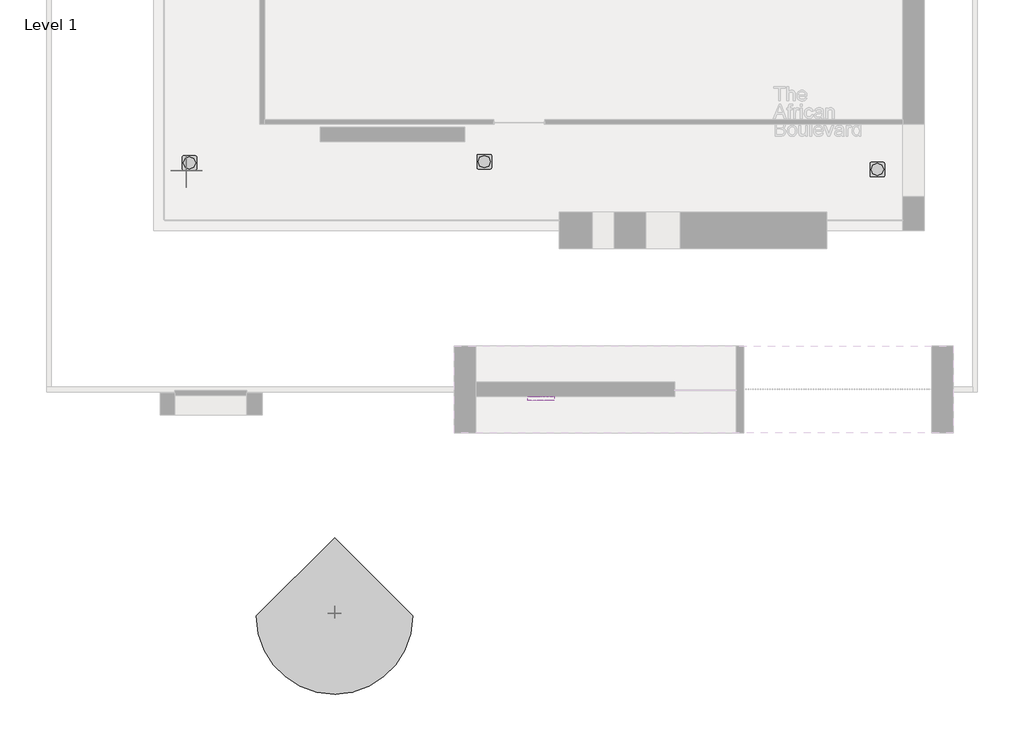
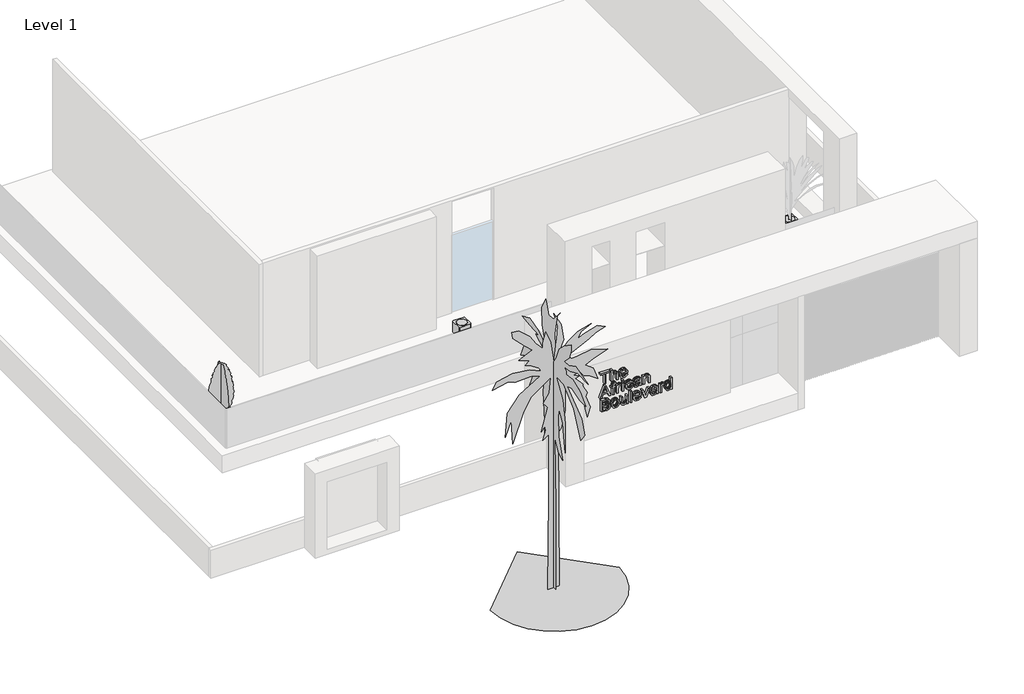
# One storey, part 2 of 3: 4 proxies, 2 geographic elements.
"""IFC4 building model written with IfcOpenShell, lengths in millimetres."""

from ifc_helpers import new_model, si_unit, frame, origin, place, context, project, spatial, polyline, outline, extrude, transform, mapped, element, save
from components import proxy_13b82c07, rpc_tree_conifer_chinese_juniper_7_5155a079, rpc_tree_tropical_cuban_royal_palm_25_0a7aa95b

model = new_model("IFC4")

# Units and contexts
model_context = context("Model", 3, world=origin())
ifc_project = project(units=[si_unit("LENGTHUNIT", "METRE", prefix="MILLI")], contexts=[model_context])

# Site, building, storey
site = spatial("IfcSite", under=ifc_project)
building = spatial("IfcBuilding", under=site)
storey = spatial("IfcBuildingStorey", under=building, Name="Level 1", Elevation=0.0)

# Proxies
placement = place(None, origin())
element("IfcBuildingElementProxy", 1, Name="24\" Arial", ObjectType="24\" Arial", at=placement, inside=storey, context=model_context, shape_type="SweptSolid", body=[
    extrude(outline(polyline([(2851.6933185, -10689.1512107), (2851.6933185, -10614.1235184), (3376.8871646, -10614.1235184), (3376.8871646, -10417.1758261), (3451.9148569, -10417.1758261), (3451.9148569, -10886.098903), (3376.8871646, -10886.098903), (3376.8871646, -10689.1512107), (2851.6933185, -10689.1512107)])), frame((0.0, -12620.7632813, 0.0), z_axis=(0.0, 1.0, 0.0), x_axis=(0.0, 0.0, 1.0)), (0.0, 0.0, 1.0), 152.4),
    extrude(outline(polyline([(2851.6933185, -10342.1481338), (2851.6933185, -10267.1204415), (3085.86178, -10267.1204415), (3130.8124531, -10264.0614511), (3164.8460108, -10254.88448), (3190.4536069, -10238.5088069), (3210.1263954, -10213.8537107), (3222.6554339, -10184.0880857), (3226.83178, -10152.3808261), (3225.2839675, -10131.718903), (3220.64053, -10113.5481338), (3212.9014675, -10097.8685184), (3202.06678, -10084.6800569), (3187.8342319, -10074.2300329), (3169.9015877, -10066.76573), (3148.2688473, -10062.2871482), (3122.9360108, -10060.7942877), (2851.6933185, -10060.7942877), (2851.6933185, -9985.7665954), (3130.7025493, -9985.7665954), (3187.6693762, -9989.61323), (3229.3229339, -10001.1531338), (3259.6380781, -10021.6318838), (3282.5896646, -10052.2950569), (3297.0420204, -10091.237653), (3301.8594723, -10136.5546723), (3297.4450012, -10174.2791675), (3284.2015877, -10208.6149607), (3262.1292319, -10239.5620521), (3231.2279339, -10267.1204415), (3451.9148569, -10267.1204415), (3451.9148569, -10342.1481338), (2851.6933185, -10342.1481338)])), frame((0.0, -12620.7632813, 0.0), z_axis=(0.0, 1.0, 0.0), x_axis=(0.0, 0.0, 1.0)), (0.0, 0.0, 1.0), 152.4),
    extrude(outline(polyline([(2982.99178, -9573.9935184), (2953.3543762, -9595.0217877), (2933.0221646, -9622.3512107), (2921.2624531, -9655.9817877), (2917.3425493, -9695.9135184), (2919.4581983, -9723.6596603), (2925.8051454, -9749.0153934), (2936.3833906, -9771.9807179), (2951.1929339, -9792.5556338), (2969.9773329, -9809.787641), (2992.4801454, -9822.7242396), (3018.7013714, -9831.3654295), (3048.6410108, -9835.7112107), (3048.6410108, -9498.5262107), (3068.8633185, -9498.0865954), (3121.1500733, -9501.6447324), (3167.2272608, -9512.3191434), (3207.094881, -9530.1098285), (3240.7529339, -9555.0167877), (3267.4870444, -9585.5288429), (3286.5828377, -9620.1348165), (3298.0403137, -9658.8347083), (3301.8594723, -9701.6285184), (3298.031155, -9745.8464992), (3286.5462031, -9785.7415954), (3267.4046166, -9821.3138069), (3240.6063954, -9852.5631338), (3206.8750733, -9878.0150329), (3166.9341839, -9896.1949607), (3120.7837271, -9907.1029175), (3068.4237031, -9910.738903), (3017.7809267, -9907.1395521), (2973.1187512, -9896.3414992), (2934.4371767, -9878.3447444), (2901.7362031, -9853.1492877), (2875.7393642, -9821.8175329), (2857.1701935, -9785.4118838), (2846.0286911, -9743.9323405), (2842.3148569, -9697.378903), (2844.4671406, -9660.1352372), (2850.9239916, -9626.3627011), (2861.6854098, -9596.0612949), (2876.7513954, -9569.2310184), (2895.7189675, -9546.1099968), (2918.1851454, -9526.936355), (2944.1499291, -9511.7100929), (2973.6133185, -9500.4312107), (2982.99178, -9573.9935184)]), holes=[polyline([(3123.6687031, -9835.7112107), (3146.0020805, -9831.6401891), (3165.9633666, -9823.3836627), (3183.5525613, -9810.9416314), (3198.7696646, -9794.3140954), (3211.0468401, -9774.4993478), (3219.8162512, -9752.4956819), (3225.0778978, -9728.3030978), (3226.83178, -9701.9215954), (3224.6337031, -9672.9985665), (3218.0394723, -9646.896403), (3207.0490877, -9623.615105), (3191.6625493, -9603.1546723), (3178.8953858, -9591.9902732), (3163.3073569, -9583.2620761), (3123.6687031, -9573.1142877), (3123.6687031, -9835.7112107)])]), frame((0.0, -12620.7632813, 0.0), z_axis=(0.0, 1.0, 0.0), x_axis=(0.0, 0.0, 1.0)), (0.0, 0.0, 1.0), 152.4),
    extrude(outline(polyline([(2110.7948569, -10908.958903), (2110.7948569, -10829.8281338), (2298.3640877, -10761.2481338), (2298.3640877, -10513.8912107), (2110.7948569, -10445.3112107), (2110.7948569, -10366.033903), (2711.0163954, -10605.4777492), (2711.0163954, -10669.3685184), (2110.7948569, -10908.958903)]), holes=[polyline([(2373.39178, -10733.698903), (2533.8513954, -10674.93698), (2635.9887031, -10637.5696723), (2520.9560108, -10595.5131338), (2373.39178, -10541.293903), (2373.39178, -10733.698903)])]), frame((0.0, -12620.7632813, 0.0), z_axis=(0.0, 1.0, 0.0), x_axis=(0.0, 0.0, 1.0)), (0.0, 0.0, 1.0), 152.4),
    extrude(outline(polyline([(2110.7948569, -10276.498903), (2110.7948569, -10201.4712107), (2476.5548569, -10201.4712107), (2476.5548569, -10117.0650569), (2551.5825493, -10117.0650569), (2551.5825493, -10201.4712107), (2586.4587031, -10201.4712107), (2615.0703377, -10198.0092396), (2632.9113954, -10187.6233261), (2642.2532223, -10168.8847204), (2645.3671646, -10140.3646723), (2641.8502416, -10097.1358261), (2712.1887031, -10086.1454415), (2718.3433185, -10122.01073), (2720.3948569, -10154.578903), (2716.1086069, -10197.5879415), (2703.2498569, -10230.1927492), (2683.5037993, -10253.4923646), (2658.5556262, -10268.5858261), (2632.7282223, -10274.5206338), (2595.9837031, -10276.498903), (2551.5825493, -10276.498903), (2551.5825493, -10342.1481338), (2476.5548569, -10342.1481338), (2476.5548569, -10276.498903), (2110.7948569, -10276.498903)])), frame((0.0, -12620.7632813, 0.0), z_axis=(0.0, 1.0, 0.0), x_axis=(0.0, 0.0, 1.0)), (0.0, 0.0, 1.0), 152.4),
    extrude(outline(polyline([(2110.7948569, -10051.4158261), (2110.7948569, -9976.3881338), (2342.4721646, -9976.3881338), (2388.1921646, -9973.3474607), (2430.1021646, -9964.2254415), (2453.4750493, -9953.363278), (2471.1329339, -9937.1890954), (2482.2332223, -9917.168278), (2485.9333185, -9894.7662107), (2482.0866839, -9868.3892877), (2470.54678, -9842.0123646), (2537.8079339, -9816.9542877), (2555.1727416, -9854.9077492), (2560.9610108, -9892.2750569), (2557.3341839, -9916.74698), (2546.4537031, -9939.1673646), (2524.1798569, -9961.51448), (2486.3729339, -9985.7665954), (2551.5825493, -9985.7665954), (2551.5825493, -10051.4158261), (2110.7948569, -10051.4158261)])), frame((0.0, -12620.7632813, 0.0), z_axis=(0.0, 1.0, 0.0), x_axis=(0.0, 0.0, 1.0)), (0.0, 0.0, 1.0), 152.4),
    extrude(outline(polyline([(-9695.0342877, -12620.7632813), (-9770.06198, -12620.7632813), (-9770.06198, -12468.3632813), (-9695.0342877, -12468.3632813), (-9695.0342877, -12620.7632813)])), frame((0.0, 0.0, 2110.7948569), z_axis=(0.0, 0.0, 1.0), x_axis=(1.0, 0.0, 0.0)), (0.0, 0.0, 1.0), 440.7876923),
    extrude(outline(polyline([(-9695.0342877, -12620.7632813), (-9770.06198, -12620.7632813), (-9770.06198, -12468.3632813), (-9695.0342877, -12468.3632813), (-9695.0342877, -12620.7632813)])), frame((0.0, 0.0, 2635.9887031), z_axis=(0.0, 0.0, 1.0), x_axis=(1.0, 0.0, 0.0)), (0.0, 0.0, 1.0), 75.0276923),
    extrude(outline(polyline([(2270.2287031, -9301.138903), (2247.8907464, -9306.2448526), (2228.6484146, -9313.9427011), (2212.5017079, -9324.2324487), (2199.4506262, -9337.1140954), (2189.3852656, -9352.1663429), (2182.1957223, -9368.9678934), (2176.4440877, -9407.818903), (2178.7474892, -9433.0097804), (2185.6576935, -9455.682028), (2197.1747007, -9475.8356458), (2213.2985108, -9493.4706338), (2234.5145324, -9507.7993478), (2261.3081743, -9518.0341434), (2293.6794363, -9524.1750208), (2331.6283185, -9526.22198), (2369.0139435, -9524.1292276), (2401.01428, -9517.8509704), (2427.6293281, -9507.3872083), (2448.8590877, -9492.7379415), (2465.0790637, -9474.745766), (2476.6647608, -9454.253278), (2483.6161791, -9431.2604776), (2485.9333185, -9405.7673646), (2481.2257704, -9372.9244319), (2467.1031262, -9345.3202492), (2443.638655, -9324.1271242), (2410.9056262, -9310.5173646), (2420.2840877, -9235.4896723), (2452.0646166, -9243.7095641), (2479.9985108, -9255.9134704), (2504.0857704, -9272.101391), (2524.3263954, -9292.2733261), (2540.3540396, -9316.0262949), (2551.8023569, -9342.9573165), (2558.6713473, -9373.066391), (2560.9610108, -9406.3535184), (2559.2941358, -9433.3944439), (2554.2935108, -9459.4187588), (2545.9591358, -9484.4264631), (2534.2910108, -9508.4175569), (2519.2845565, -9530.3983261), (2500.9351935, -9549.3750569), (2479.2429218, -9565.3477492), (2454.2077416, -9578.316403), (2426.3883305, -9588.3497083), (2396.3433666, -9595.516355), (2329.57678, -9601.2496723), (2277.679268, -9597.8930256), (2232.183655, -9587.8230857), (2193.0899411, -9571.0398526), (2160.3981262, -9547.5433261), (2134.593619, -9518.5149728), (2116.1618281, -9485.1362588), (2105.1027536, -9447.4071843), (2101.4163954, -9405.3277492), (2104.058667, -9371.4590473), (2111.9854819, -9340.3379415), (2125.1968401, -9311.9644319), (2143.6927416, -9286.3385184), (2166.8687151, -9264.3852252), (2194.1202896, -9247.0295761), (2225.4474651, -9234.2715713), (2260.8502416, -9226.1112107), (2270.2287031, -9301.138903)])), frame((0.0, -12620.7632813, 0.0), z_axis=(0.0, 1.0, 0.0), x_axis=(0.0, 0.0, 1.0)), (0.0, 0.0, 1.0), 152.4),
    extrude(outline(polyline([(2167.0656262, -8879.1081338), (2136.8787031, -8872.3673646), (2110.7948569, -8860.3512107), (2110.7948569, -8785.3235184), (2141.6595204, -8794.6287107), (2173.8796646, -8800.2704415), (2304.2256262, -8804.0804415), (2397.5706262, -8804.0804415), (2463.2198569, -8807.743903), (2491.3369243, -8816.792653), (2514.1419723, -8830.7504415), (2532.5875012, -8851.797028), (2547.6260108, -8882.1121723), (2557.6272608, -8922.3186627), (2560.9610108, -8973.0392877), (2557.1876454, -9025.921355), (2545.8675493, -9072.0260184), (2527.5868762, -9109.7230377), (2502.93178, -9137.3821723), (2470.6933185, -9156.8168357), (2429.6625493, -9169.8404415), (2420.2840877, -9094.8127492), (2451.4784627, -9079.9024607), (2471.49928, -9058.6177492), (2482.3248089, -9027.4050569), (2485.9333185, -8982.7108261), (2480.5113954, -8934.426403), (2473.7339916, -8915.3947204), (2464.2456262, -8899.7700569), (2454.7389435, -8890.7304655), (2442.3381262, -8884.2736146), (2408.8540877, -8879.1081338), (2392.1487031, -8879.5477492), (2378.2275493, -8932.9610184), (2366.3579339, -9009.673903), (2355.0744723, -9074.5904415), (2344.7435108, -9102.304528), (2330.4560108, -9127.12448), (2311.5525493, -9148.2443357), (2287.3737031, -9164.8581338), (2259.1284146, -9175.6287107), (2228.0256262, -9179.218903), (2201.5662752, -9176.8422324), (2177.5797608, -9169.7122204), (2156.0660829, -9157.828867), (2137.0252416, -9141.1921723), (2121.4463714, -9120.1226891), (2110.3186069, -9094.9409704), (2103.6419483, -9065.647016), (2101.4163954, -9032.2408261), (2105.1164916, -8990.678855), (2116.21678, -8951.86448), (2136.3291839, -8914.955105), (2167.0656262, -8879.1081338)]), holes=[polyline([(2317.1210108, -8879.1081338), (2295.8729339, -8879.5477492), (2262.1690877, -8882.515153), (2237.8437031, -8891.4173646), (2214.2326935, -8911.4931338), (2194.3950493, -8940.3612107), (2180.9318281, -8975.9700569), (2176.4440877, -9016.2681338), (2180.51053, -9054.2765473), (2192.7098569, -9081.8440954), (2210.99053, -9098.6044319), (2233.3010108, -9104.1912107), (2248.4311069, -9101.6267877), (2262.1690877, -9093.9335184), (2273.6357223, -9081.4960665), (2281.95178, -9064.6990954), (2294.1144723, -9000.148903), (2304.6286069, -8929.5173646), (2317.1210108, -8879.1081338)])]), frame((0.0, -12620.7632813, 0.0), z_axis=(0.0, 1.0, 0.0), x_axis=(0.0, 0.0, 1.0)), (0.0, 0.0, 1.0), 152.4),
    extrude(outline(polyline([(2110.7948569, -8700.9173646), (2110.7948569, -8625.8896723), (2344.6702416, -8625.8896723), (2382.5412752, -8623.7511266), (2413.7997608, -8617.3354896), (2438.4456983, -8606.6427612), (2456.4790877, -8591.6729415), (2469.3653137, -8573.7540353), (2478.5697608, -8554.2140473), (2484.0924291, -8533.0529776), (2485.9333185, -8510.2708261), (2482.6545204, -8482.5933742), (2472.8181262, -8458.7625569), (2457.4865396, -8440.1704896), (2437.7221646, -8428.2092877), (2410.1362993, -8421.7249607), (2371.3402416, -8419.5635184), (2110.7948569, -8419.5635184), (2110.7948569, -8344.5358261), (2381.4513954, -8344.5358261), (2453.9879339, -8348.4923646), (2483.7535589, -8357.3396242), (2509.1596646, -8370.9860184), (2530.1512993, -8391.0984223), (2546.6735108, -8419.3437107), (2557.3891358, -8453.2124127), (2560.9610108, -8490.1950569), (2556.5282223, -8531.9768357), (2543.2298569, -8568.5198646), (2521.0659146, -8599.8241434), (2490.0363954, -8625.8896723), (2551.5825493, -8625.8896723), (2551.5825493, -8700.9173646), (2110.7948569, -8700.9173646)])), frame((0.0, -12620.7632813, 0.0), z_axis=(0.0, 1.0, 0.0), x_axis=(0.0, 0.0, 1.0)), (0.0, 0.0, 1.0), 152.4),
    extrude(outline(polyline([(1369.8963954, -10839.2065954), (1369.8963954, -10611.9254415), (1372.4791358, -10559.3730857), (1380.2273569, -10515.7229415), (1393.0128377, -10479.8027011), (1410.7073569, -10450.4400569), (1435.1426454, -10426.4627011), (1468.1504339, -10406.6983261), (1506.9648089, -10393.4549127), (1548.8198569, -10389.0404415), (1574.8212752, -10390.6569439), (1599.0459146, -10395.5064511), (1621.4937752, -10403.5889631), (1642.1648569, -10414.90448), (1660.5004819, -10429.2240353), (1675.9419723, -10446.3186627), (1688.4893281, -10466.1883622), (1698.1425493, -10488.8331338), (1721.5337512, -10453.242605), (1751.2627416, -10427.946403), (1785.2413473, -10412.8346242), (1821.3813954, -10407.7973646), (1860.6537031, -10413.7871242), (1898.1675493, -10431.756403), (1915.2988113, -10444.880754), (1930.0579819, -10460.2947684), (1942.4450613, -10477.9984463), (1952.4600493, -10497.9917877), (1965.7034627, -10547.1737588), (1970.1179339, -10610.16698), (1970.1179339, -10839.2065954), (1369.8963954, -10839.2065954)]), holes=[polyline([(1726.2779339, -10764.178903), (1895.0902416, -10764.178903), (1895.0902416, -10637.5696723), (1893.1302896, -10579.3206338), (1887.2504339, -10541.1473646), (1876.0951935, -10516.2724607), (1858.3090877, -10497.9185184), (1835.5223569, -10486.5984223), (1809.3652416, -10482.8250569), (1782.4204819, -10486.8731819), (1760.4946646, -10499.0175569), (1743.8442319, -10519.148278), (1732.7256262, -10547.1554415), (1727.8898569, -10579.2473646), (1726.2779339, -10627.1654415), (1726.2779339, -10764.178903)]), polyline([(1444.9240877, -10764.178903), (1651.2502416, -10764.178903), (1651.2502416, -10617.6404415), (1648.7407704, -10564.208855), (1641.2123569, -10524.9548646), (1627.4926935, -10497.240778), (1606.4094723, -10478.428903), (1579.4463954, -10467.6583261), (1548.0871646, -10464.0681338), (1521.0874531, -10467.1271242), (1497.5313954, -10476.3040954), (1478.279905, -10490.2252492), (1464.1938954, -10507.5167877), (1454.3575012, -10528.7831819), (1447.8548569, -10554.628903), (1444.9240877, -10610.3135184), (1444.9240877, -10764.178903)])]), frame((0.0, -12620.7632813, 0.0), z_axis=(0.0, 1.0, 0.0), x_axis=(0.0, 0.0, 1.0)), (0.0, 0.0, 1.0), 152.4),
    extrude(outline(polyline([(1590.2902416, -10314.0127492), (1537.8661069, -10310.6103093), (1491.9629339, -10300.4029896), (1452.5807223, -10283.3907901), (1419.7194723, -10259.5737107), (1393.8187993, -10230.2431218), (1375.3183185, -10196.6903934), (1364.21803, -10158.9155256), (1360.5179339, -10116.9185184), (1362.1985468, -10089.9050689), (1367.2403858, -10063.9631819), (1375.6434507, -10039.0928574), (1387.4077416, -10015.2940954), (1402.2127055, -9993.4186506), (1419.7377896, -9974.318278), (1439.982994, -9957.9929776), (1462.9483185, -9944.4427492), (1489.5358906, -9933.8003934), (1520.6478377, -9926.1987107), (1556.2841598, -9921.6377011), (1596.4448569, -9920.1173646), (1645.9977536, -9923.5564391), (1689.8814435, -9933.8736627), (1728.0959267, -9951.0690353), (1760.6412031, -9975.1425569), (1786.638042, -10004.6380016), (1805.2072127, -10038.0991434), (1816.3487151, -10075.5259824), (1820.0625493, -10116.9185184), (1817.0127175, -10154.4140473), (1807.8632223, -10188.9421723), (1792.6140637, -10220.5028934), (1771.2652416, -10249.0962107), (1737.863631, -10277.4971963), (1696.5672608, -10297.7836146), (1647.376131, -10309.9554655), (1590.2902416, -10314.0127492)]), holes=[polyline([(1590.43678, -10238.9850569), (1626.8195324, -10236.8144559), (1658.302405, -10230.302653), (1684.8853978, -10219.4496482), (1706.5685108, -10204.2554415), (1723.3975372, -10185.773278), (1735.4182704, -10165.056403), (1742.6307103, -10142.1048165), (1745.0348569, -10116.9185184), (1742.6215517, -10092.0390353), (1735.3816358, -10069.2752011), (1723.3151093, -10048.627016), (1706.4219723, -10030.09448), (1684.8396045, -10014.8041074), (1658.7053858, -10003.8824127), (1628.0193161, -9997.3293958), (1592.7813954, -9995.1450569), (1555.5423089, -9997.3156579), (1523.3954339, -10003.8274607), (1496.3407704, -10014.6804655), (1474.3783185, -10029.8746723), (1457.3890156, -10048.3385184), (1445.2537993, -10069.0004415), (1437.9726694, -10091.8604415), (1435.5456262, -10116.9185184), (1437.9589315, -10142.1048165), (1445.1988473, -10165.056403), (1457.2653738, -10185.773278), (1474.1585108, -10204.2554415), (1495.9057343, -10219.4496482), (1522.5345204, -10230.302653), (1554.044869, -10236.8144559), (1590.43678, -10238.9850569)])]), frame((0.0, -12620.7632813, 0.0), z_axis=(0.0, 1.0, 0.0), x_axis=(0.0, 0.0, 1.0)), (0.0, 0.0, 1.0), 152.4),
    extrude(outline(polyline([(1369.8963954, -9554.3573646), (1369.8963954, -9479.3296723), (1810.6840877, -9479.3296723), (1810.6840877, -9554.3573646), (1581.3513954, -9554.3573646), (1533.048655, -9557.3980377), (1497.7512031, -9566.5200569), (1471.9787512, -9582.9506819), (1452.2510108, -9607.9171723), (1439.7219723, -9638.1956819), (1435.5456262, -9670.5623646), (1439.6303858, -9701.1705857), (1451.8846646, -9726.4667877), (1471.2826935, -9745.2053934), (1496.7987031, -9756.1408261), (1525.8133185, -9759.5478454), (1573.29178, -9760.6835184), (1810.6840877, -9760.6835184), (1810.6840877, -9835.7112107), (1537.9760108, -9835.7112107), (1468.2237031, -9831.3150569), (1438.0734146, -9822.5044319), (1412.9787031, -9808.9679415), (1392.31678, -9788.8555377), (1375.4648569, -9760.3171723), (1364.2546646, -9726.3019319), (1360.5179339, -9689.758903), (1365.8391118, -9649.2043838), (1381.8026454, -9613.1192877), (1408.4085348, -9581.5036146), (1445.65678, -9554.3573646), (1369.8963954, -9554.3573646)])), frame((0.0, -12620.7632813, 0.0), z_axis=(0.0, 1.0, 0.0), x_axis=(0.0, 0.0, 1.0)), (0.0, 0.0, 1.0), 152.4),
    extrude(outline(polyline([(-9301.138903, -12620.7632813), (-9376.1665954, -12620.7632813), (-9376.1665954, -12468.3632813), (-9301.138903, -12468.3632813), (-9301.138903, -12620.7632813)])), frame((0.0, 0.0, 1369.8963954), z_axis=(0.0, 0.0, 1.0), x_axis=(1.0, 0.0, 0.0)), (0.0, 0.0, 1.0), 600.2215385),
    extrude(outline(polyline([(1501.1948569, -8879.9873646), (1471.5574531, -8901.0156338), (1451.2252416, -8928.3450569), (1439.46553, -8961.9756338), (1435.5456262, -9001.9073646), (1437.6612752, -9029.6535064), (1444.0082223, -9055.0092396), (1454.5864675, -9077.9745641), (1469.3960108, -9098.54948), (1488.1804098, -9115.7814872), (1510.6832223, -9128.7180857), (1536.9044483, -9137.3592756), (1566.8440877, -9141.7050569), (1566.8440877, -8804.5200569), (1587.0663954, -8804.0804415), (1639.3531502, -8807.6385785), (1685.4303377, -8818.3129896), (1725.2979579, -8836.1036747), (1758.9560108, -8861.0106338), (1785.6901214, -8891.5226891), (1804.7859146, -8926.1286627), (1816.2433906, -8964.8285545), (1820.0625493, -9007.6223646), (1816.2342319, -9051.8403454), (1804.74928, -9091.7354415), (1785.6076935, -9127.307653), (1758.8094723, -9158.55698), (1725.0781502, -9184.008879), (1685.1372608, -9202.1888069), (1638.9868041, -9213.0967636), (1586.62678, -9216.7327492), (1535.9840036, -9213.1333982), (1491.3218281, -9202.3353454), (1452.6402536, -9184.3385905), (1419.93928, -9159.1431338), (1393.9424411, -9127.811379), (1375.3732704, -9091.40573), (1364.231768, -9049.9261867), (1360.5179339, -9003.3727492), (1362.6702175, -8966.1290833), (1369.1270685, -8932.3565473), (1379.8884868, -8902.055141), (1394.9544723, -8875.2248646), (1413.9220444, -8852.1038429), (1436.3882223, -8832.9302011), (1462.353006, -8817.7039391), (1491.8163954, -8806.4250569), (1501.1948569, -8879.9873646)]), holes=[polyline([(1641.87178, -9141.7050569), (1664.2051574, -9137.6340353), (1684.1664435, -9129.3775088), (1701.7556382, -9116.9354776), (1716.9727416, -9100.3079415), (1729.249917, -9080.4931939), (1738.0193281, -9058.489528), (1743.2809747, -9034.2969439), (1745.0348569, -9007.9154415), (1742.83678, -8978.9924127), (1736.2425493, -8952.8902492), (1725.2521646, -8929.6089511), (1709.8656262, -8909.1485184), (1697.0984627, -8897.9841194), (1681.5104339, -8889.2559223), (1641.87178, -8879.1081338), (1641.87178, -9141.7050569)])]), frame((0.0, -12620.7632813, 0.0), z_axis=(0.0, 1.0, 0.0), x_axis=(0.0, 0.0, 1.0)), (0.0, 0.0, 1.0), 152.4),
    extrude(outline(polyline([(1369.8963954, -8620.6142877), (1369.8963954, -8525.803903), (1810.6840877, -8372.6712107), (1810.6840877, -8452.0950569), (1541.6394723, -8546.6123646), (1457.8194723, -8574.3081338), (1546.62178, -8602.5900569), (1810.6840877, -8696.6677492), (1810.6840877, -8775.9450569), (1369.8963954, -8620.6142877)])), frame((0.0, -12620.7632813, 0.0), z_axis=(0.0, 1.0, 0.0), x_axis=(0.0, 0.0, 1.0)), (0.0, 0.0, 1.0), 152.4),
    extrude(outline(polyline([(1426.1671646, -8025.6681338), (1395.9802416, -8018.9273646), (1369.8963954, -8006.9112107), (1369.8963954, -7931.8835184), (1400.7610589, -7941.1887107), (1432.9812031, -7946.8304415), (1563.3271646, -7950.6404415), (1656.6721646, -7950.6404415), (1722.3213954, -7954.303903), (1750.4384627, -7963.352653), (1773.2435108, -7977.3104415), (1791.6890396, -7998.357028), (1806.7275493, -8028.6721723), (1816.7287993, -8068.8786627), (1820.0625493, -8119.5992877), (1816.2891839, -8172.481355), (1804.9690877, -8218.5860184), (1786.6884146, -8256.2830377), (1762.0333185, -8283.9421723), (1729.7948569, -8303.3768357), (1688.7640877, -8316.4004415), (1679.3856262, -8241.3727492), (1710.5800012, -8226.4624607), (1730.6008185, -8205.1777492), (1741.4263473, -8173.9650569), (1745.0348569, -8129.2708261), (1739.6129339, -8080.986403), (1732.83553, -8061.9547204), (1723.3471646, -8046.3300569), (1713.8404819, -8037.2904655), (1701.4396646, -8030.8336146), (1667.9556262, -8025.6681338), (1651.2502416, -8026.1077492), (1637.3290877, -8079.5210184), (1625.4594723, -8156.233903), (1614.1760108, -8221.1504415), (1603.8450493, -8248.864528), (1589.5575493, -8273.68448), (1570.6540877, -8294.8043357), (1546.4752416, -8311.4181338), (1518.2299531, -8322.1887107), (1487.1271646, -8325.778903), (1460.6678137, -8323.4022324), (1436.6812993, -8316.2722204), (1415.1676214, -8304.388867), (1396.12678, -8287.7521723), (1380.5479098, -8266.6826891), (1369.4201454, -8241.5009704), (1362.7434868, -8212.207016), (1360.5179339, -8178.8008261), (1364.21803, -8137.238855), (1375.3183185, -8098.42448), (1395.4307223, -8061.515105), (1426.1671646, -8025.6681338)]), holes=[polyline([(1576.2225493, -8025.6681338), (1554.9744723, -8026.1077492), (1521.2706262, -8029.075153), (1496.9452416, -8037.9773646), (1473.3342319, -8058.0531338), (1453.4965877, -8086.9212107), (1440.0333666, -8122.5300569), (1435.5456262, -8162.8281338), (1439.6120685, -8200.8365473), (1451.8113954, -8228.4040954), (1470.0920685, -8245.1644319), (1492.4025493, -8250.7512107), (1507.5326454, -8248.1867877), (1521.2706262, -8240.4935184), (1532.7372608, -8228.0560665), (1541.0533185, -8211.2590954), (1553.2160108, -8146.708903), (1563.7301454, -8076.0773646), (1576.2225493, -8025.6681338)])]), frame((0.0, -12620.7632813, 0.0), z_axis=(0.0, 1.0, 0.0), x_axis=(0.0, 0.0, 1.0)), (0.0, 0.0, 1.0), 152.4),
    extrude(outline(polyline([(1369.8963954, -7847.4773646), (1369.8963954, -7772.4496723), (1601.5737031, -7772.4496723), (1647.2937031, -7769.4089992), (1689.2037031, -7760.28698), (1712.5765877, -7749.4248165), (1730.2344723, -7733.2506338), (1741.3347608, -7713.2298165), (1745.0348569, -7690.8277492), (1741.1882223, -7664.4508261), (1729.6483185, -7638.073903), (1796.9094723, -7613.0158261), (1814.27428, -7650.9692877), (1820.0625493, -7688.3365954), (1816.4357223, -7712.8085184), (1805.5552416, -7735.228903), (1783.2813954, -7757.5760184), (1745.4744723, -7781.8281338), (1810.6840877, -7781.8281338), (1810.6840877, -7847.4773646), (1369.8963954, -7847.4773646)])), frame((0.0, -12620.7632813, 0.0), z_axis=(0.0, 1.0, 0.0), x_axis=(0.0, 0.0, 1.0)), (0.0, 0.0, 1.0), 152.4),
    extrude(outline(polyline([(1369.8963954, -7294.1481338), (1369.8963954, -7219.1204415), (1970.1179339, -7219.1204415), (1970.1179339, -7294.1481338), (1746.5002416, -7294.1481338), (1776.1193281, -7316.0189992), (1799.6204339, -7343.5315954), (1814.9520204, -7375.9898646), (1820.0625493, -7412.6977492), (1818.2766118, -7438.5205737), (1812.9187993, -7463.0886627), (1803.9891118, -7486.402016), (1791.4875493, -7508.4606338), (1775.6339194, -7528.5547204), (1756.64803, -7545.97448), (1734.529881, -7560.7199127), (1709.2794723, -7572.7910184), (1652.6057223, -7588.8919319), (1589.8506262, -7594.258903), (1526.3078858, -7588.4339992), (1497.4352295, -7581.1528694), (1470.4950493, -7570.9592877), (1445.9544363, -7558.118855), (1424.2804819, -7542.8971723), (1405.4731863, -7525.2942396), (1389.5325493, -7505.3100569), (1376.838655, -7483.6223646), (1367.7715877, -7460.908903), (1362.3313473, -7437.1696723), (1360.5179339, -7412.4046723), (1365.5277175, -7375.7242636), (1380.5570685, -7343.7880377), (1405.6059868, -7316.5959944), (1440.6744723, -7294.1481338), (1369.8963954, -7294.1481338)]), holes=[polyline([(1590.1437031, -7519.2312107), (1627.6071767, -7517.2529415), (1659.6945204, -7511.3181338), (1686.4057343, -7501.4267877), (1707.7408185, -7487.578903), (1724.0569603, -7470.7727732), (1735.7113473, -7452.0066915), (1742.7039795, -7431.2806579), (1745.0348569, -7408.5946723), (1742.6078137, -7385.3729054), (1735.3266839, -7364.0652973), (1723.1914675, -7344.6718478), (1706.2021646, -7327.1925569), (1684.0290637, -7312.7356218), (1656.3424531, -7302.4092396), (1623.1423329, -7296.2134103), (1584.4287031, -7294.1481338), (1549.1175132, -7296.1767756), (1518.6512512, -7302.2627011), (1493.029917, -7312.4059103), (1472.2535108, -7326.606403), (1456.1938113, -7343.7101891), (1444.7225973, -7362.563278), (1437.839869, -7383.1656699), (1435.5456262, -7405.5173646), (1437.9497728, -7427.7637348), (1445.1622127, -7448.4897684), (1457.1829459, -7467.6954655), (1474.0119723, -7485.3808261), (1495.6950853, -7500.1903694), (1522.2780781, -7510.7686146), (1553.7609507, -7517.1155617), (1590.1437031, -7519.2312107)])]), frame((0.0, -12620.7632813, 0.0), z_axis=(0.0, 1.0, 0.0), x_axis=(0.0, 0.0, 1.0)), (0.0, 0.0, 1.0), 152.4),
])
proxy_shape = proxy_13b82c07(model_context)
element("IfcBuildingElementProxy", 2, Name="Air Conditioner-Outside Unit : 33\" x 24\" x 24\"", ObjectType="Air Conditioner-Outside Unit : 33\" x 24\" x 24\"", at=placement, inside=storey, context=model_context, shape_type="MappedRepresentation", body=[
    mapped(proxy_shape, transform((-24603.5874719, -2613.1632813, 0.0), x_axis=(1.0, 0.0, 0.0), y_axis=(0.0, 1.0, 0.0), z_axis=(0.0, 0.0, 1.0))),
])
element("IfcBuildingElementProxy", 3, Name="Air Conditioner-Outside Unit : 33\" x 24\" x 24\"", ObjectType="Air Conditioner-Outside Unit : 33\" x 24\" x 24\"", at=placement, inside=storey, context=model_context, shape_type="MappedRepresentation", body=[
    mapped(proxy_shape, transform((4377.8125281, -2892.5632813, 0.0), x_axis=(1.0, 0.0, 0.0), y_axis=(0.0, 1.0, 0.0), z_axis=(0.0, 0.0, 1.0))),
])
element("IfcBuildingElementProxy", 4, Name="Air Conditioner-Outside Unit : 33\" x 24\" x 24\"", ObjectType="Air Conditioner-Outside Unit : 33\" x 24\" x 24\"", at=placement, inside=storey, context=model_context, shape_type="MappedRepresentation", body=[
    mapped(proxy_shape, transform((-12182.9874719, -2562.3632813, 0.0), x_axis=(1.0, 0.0, 0.0), y_axis=(0.0, 1.0, 0.0), z_axis=(0.0, 0.0, 1.0))),
])

# Geographic elements
rpc_tree_conifer_chinese_juniper_7_shape = rpc_tree_conifer_chinese_juniper_7_5155a079(model_context)
element("IfcGeographicElement", 5, ObjectType="RPC Tree - Conifer : Chinese Juniper - 7'", at=placement, inside=storey, context=model_context, shape_type="MappedRepresentation", body=[
    mapped(rpc_tree_conifer_chinese_juniper_7_shape, transform((-24730.784143, -2943.3632813, 0.0), x_axis=(1.0, 0.0, 0.0), y_axis=(0.0, 1.0, 0.0), z_axis=(0.0, 0.0, 1.0))),
])
rpc_tree_tropical_cuban_royal_palm_25_shape = rpc_tree_tropical_cuban_royal_palm_25_0a7aa95b(model_context)
element("IfcGeographicElement", 6, ObjectType="RPC Tree - Tropical : Cuban Royal Palm - 25'", at=placement, inside=storey, context=model_context, shape_type="MappedRepresentation", body=[
    mapped(rpc_tree_tropical_cuban_royal_palm_25_shape, transform((-18482.1874719, -21612.3632813, 0.0), x_axis=(1.0, 0.0, 0.0), y_axis=(0.0, 1.0, 0.0), z_axis=(0.0, 0.0, 1.0))),
])

save(model, "model.ifc")

# Revit data of these elements
# Type "Air Conditioner-Outside Unit : 33\" x 24\" x 24\""
#   Assembly Code = "D3030"
#   Depth = 2' - 0"
#   Height = 2' - 0"
#   Width = 2' - 0"
#   Air Conditioner Material = Steel, Paint Finish, Dark Gray, Matte
#   Default Elevation = 0
# Type "RPC Tree - Conifer : Chinese Juniper - 7'"
#   built-in parameter 1005198 = "{2, 15},{39, RPC-16-FUM3-UUQ0-UBF0-N000-ST1L-LVER-AU},{1, 0},{1, 0},{2, 13},{1, 8},{5, Color},{1, 0},{1, 0},{3, 0.8},{3, 0.8},{3, 0.8},{1, 8},{7, BBoxMin},{1, 0},{1, 0},{1, 0},{1, 0},{1, 0},{1, 8},{7, BBoxMax},{1, 0},{1, 0},{1, 0},{1, 0},{1, 0},{2, 11},{9, RPCTypeId},{1, 0},{1, 0},{39, RPC-16-FUM3-UUQ0-UBF0-N000-ST1L-LVER-AU},{1, 6},{14, RPCPlantHeight},{1, 0},{1, 0},{1, 7},{2, 11},{7, keyword},{1, 0},{1, 0},{34, :RPCs:Trees [General]:Geometry:RPC},{2, 11},{8, category},{1, 0},{1, 0},{15, Trees [General]},{2, 11},{12, LocalizedUID},{1, 0},{1, 0},{15, Chinese Juniper},{2, 14},{6, Height},{1, 0},{1, 0},{1, 7},{1, 2},{16, Cast Reflections},{1, 0},{1, 0},{1, 0},{1, 2},{12, Cast Shadows},{1, 0},{1, 0},{1, 1},{1, 2},{9, Lock View},{1, 0},{1, 0},{1, 0},{1, 4},{5, ViewC},{1, 0},{1, 0},{1, 0},{21, assetlibrary_base.fbx},{1, 5},"
#   built-in parameter 1005195 = "RPC-16-FUM3-UUQ0-UBF0-N000-ST1L-LVER-AU"
#   Type Comments = "Chinese Juniper"
#   Assembly Code = "G2050500"
#   Height = 10' - 0"
#   Description = (empty or 0)
#   Default Elevation = 0
# Type "RPC Tree - Tropical : Cuban Royal Palm - 25'"
#   built-in parameter 1005198 = "{2, 15},{39, RPC-16-FVGV-NKG0-7NHH-C000-ST1L-LVER-AU},{1, 0},{1, 0},{2, 13},{1, 8},{5, Color},{1, 0},{1, 0},{3, 0.8},{3, 0.8},{3, 0.8},{1, 8},{7, BBoxMin},{1, 0},{1, 0},{1, 0},{1, 0},{1, 0},{1, 8},{7, BBoxMax},{1, 0},{1, 0},{1, 0},{1, 0},{1, 0},{2, 11},{9, RPCTypeId},{1, 0},{1, 0},{39, RPC-16-FVGV-NKG0-7NHH-C000-ST1L-LVER-AU},{1, 6},{14, RPCPlantHeight},{1, 0},{1, 0},{2, 25},{2, 11},{7, keyword},{1, 0},{1, 0},{35, :RPCs:Trees [Tropical]:Geometry:RPC},{2, 11},{8, category},{1, 0},{1, 0},{16, Trees [Tropical]},{2, 11},{12, LocalizedUID},{1, 0},{1, 0},{16, Cuban Royal Palm},{2, 14},{6, Height},{1, 0},{1, 0},{2, 25},{1, 2},{16, Cast Reflections},{1, 0},{1, 0},{1, 0},{1, 2},{12, Cast Shadows},{1, 0},{1, 0},{1, 1},{1, 2},{9, Lock View},{1, 0},{1, 0},{1, 0},{1, 4},{5, ViewC},{1, 0},{1, 0},{1, 0},{21, assetlibrary_base.fbx},{1, 5},"
#   built-in parameter 1005195 = "RPC-16-FVGV-NKG0-7NHH-C000-ST1L-LVER-AU"
#   Type Comments = "Cuban Royal Palm"
#   Assembly Code = "G2050500"
#   Height = 50' - 0"
#   Plan Symbol = element 321958
#   Default Elevation = 0
# Element 1 (IfcBuildingElementProxy, "24\" Arial")
#   Phase Created = New Construction
# Element 2 (IfcBuildingElementProxy, "Air Conditioner-Outside Unit : 33\" x 24\" x 24\"")
#   Mark = "1"
#   Phase Created = New Construction
#   Materials on its faces: "Steel, Paint Finish, Dark Gray, Matte"
# Element 3 (IfcBuildingElementProxy, "Air Conditioner-Outside Unit : 33\" x 24\" x 24\"")
#   Mark = "2"
#   Phase Created = New Construction
#   Materials on its faces: "Steel, Paint Finish, Dark Gray, Matte"
# Element 4 (IfcBuildingElementProxy, "Air Conditioner-Outside Unit : 33\" x 24\" x 24\"")
#   Mark = "3"
#   Phase Created = New Construction
#   Materials on its faces: "Steel, Paint Finish, Dark Gray, Matte"
# Element 5 (IfcGeographicElement, "RPC Tree - Conifer : Chinese Juniper - 7'")
#   Phase Created = New Construction
# Element 6 (IfcGeographicElement, "RPC Tree - Tropical : Cuban Royal Palm - 25'")
#   Phase Created = New Construction
# Materials
#   "Steel, Paint Finish, Dark Gray, Matte": class "Metal", colour RGB 98 98 98, transparency 0, Description = "Steel, paint finish, dark gray, matte", Cost = 0
